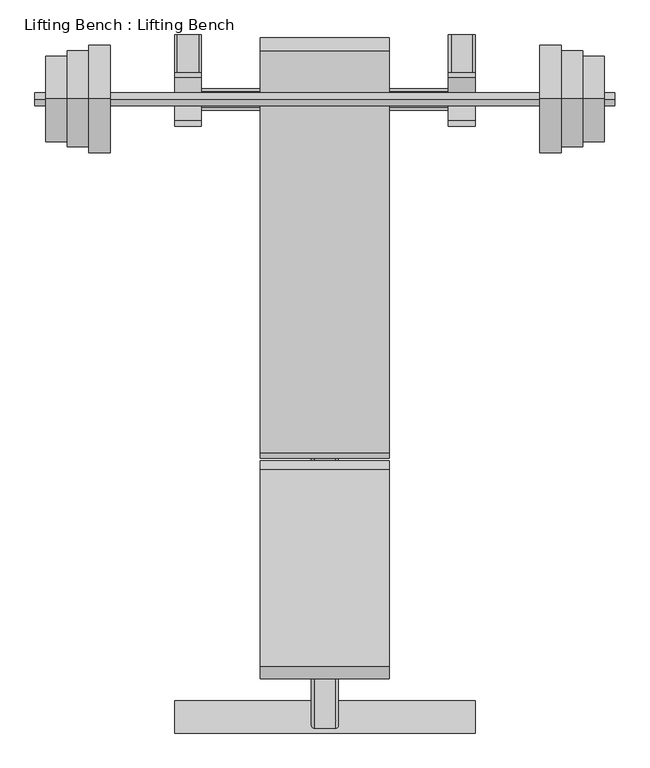
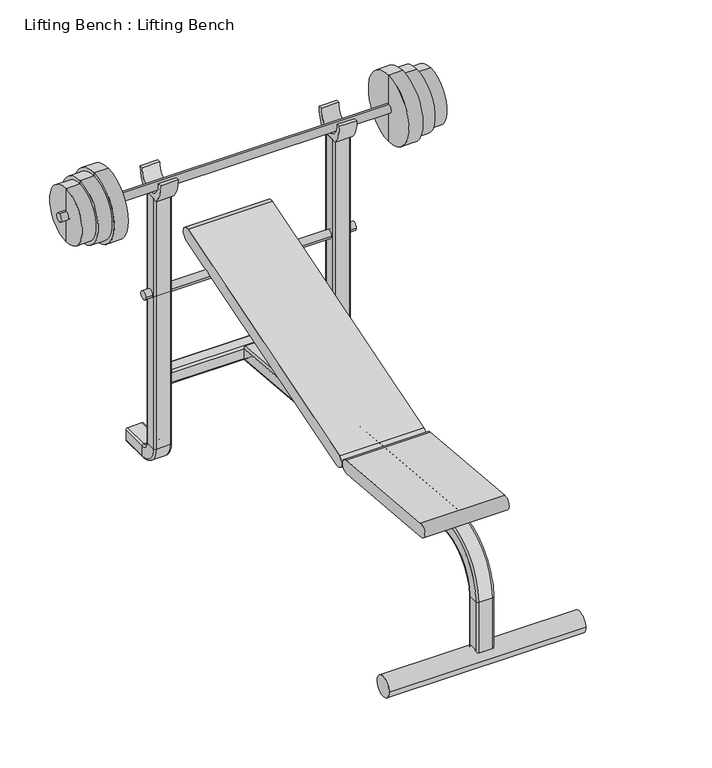
"""IFC4 building model written with IfcOpenShell, lengths in millimetres: proxy geometry, Lifting Bench : Lifting Bench."""

from ifc_helpers import new_model, si_unit, point, frame, frame_2d, origin, place, context, project, spatial, polyline, circle_curve, ellipse_curve, trimmed, segment, composite_curve, outline, extrude, source, transform, mapped, element, save
from ifc_brep_helpers import plane_surface, cylinder_surface, revolved_surface, advanced_brep


def lifting_bench_lifting_bench_243d69f3(model_context):
    return source(origin(), model_context, "Body", "SolidModel", [
        extrude(outline(composite_curve([segment(trimmed(circle_curve(frame_2d((38.1, 39.9587999)), 38.1), [point((0.0, 39.9587999))], [point((76.2, 39.9587999))], False, "CARTESIAN"), True, "CONTINUOUS"), segment(trimmed(circle_curve(frame_2d((38.1, 39.9587999)), 38.1), [point((76.2, 39.9587999))], [point((0.0, 39.9587999))], False, "CARTESIAN"), True, "CONTINUOUS")], self_intersect=False)), frame((0.0, 0.0, 0.0), z_axis=(1.0, 0.0, 0.0), x_axis=(0.0, 1.0, 0.0)), (0.0, 0.0, 1.0), 711.2),
        advanced_brep(
        [(57.15, 1524.0, 1033.9133719), (6.35, 1524.0, 1033.9133719), (0.0, 1517.65, 1033.9133719), (0.0, 1479.55, 1033.9133719), (6.35, 1473.2, 1033.9133719), (57.15, 1473.2, 1033.9133719), (63.5, 1479.55, 1033.9133719), (63.5, 1517.65, 1033.9133719), (57.15, 1524.0, 76.2), (6.35, 1524.0, 76.2), (0.0, 1517.65, 76.2), (0.0, 1479.55, 76.2), (6.35, 1473.2, 76.2), (57.15, 1473.2, 76.2), (63.5, 1479.55, 76.2), (63.5, 1517.65, 76.2), (6.35, 1549.4, 50.8), (57.15, 1549.4, 50.8), (0.0, 1549.4, 44.45), (0.0, 1549.4, 6.35), (6.35, 1549.4, 0.0), (57.15, 1549.4, 0.0), (63.5, 1549.4, 6.35), (63.5, 1549.4, 44.45), (57.15, 1651.0, 50.8), (63.5, 1651.0, 44.45), (63.5, 1651.0, 6.35), (57.15, 1651.0, 0.0), (6.35, 1651.0, 0.0), (0.0, 1651.0, 6.35), (0.0, 1651.0, 44.45), (6.35, 1651.0, 50.8)],
        [
            (0, 1),
            (1, 2, circle_curve(frame((6.35, 1517.65, 1033.9133719), z_axis=(0.0, 0.0, 1.0), x_axis=(1.0, 0.0, 0.0)), 6.35)),
            (2, 3),
            (3, 4, circle_curve(frame((6.35, 1479.55, 1033.9133719), z_axis=(0.0, 0.0, 1.0), x_axis=(1.0, 0.0, 0.0)), 6.35)),
            (4, 5),
            (5, 6, circle_curve(frame((57.15, 1479.55, 1033.9133719), z_axis=(0.0, 0.0, 1.0), x_axis=(1.0, 0.0, 0.0)), 6.35)),
            (6, 7),
            (7, 0, circle_curve(frame((57.15, 1517.65, 1033.9133719), z_axis=(0.0, 0.0, 1.0), x_axis=(1.0, 0.0, 0.0)), 6.35)),
            (0, 8),
            (8, 9),
            (9, 1),
            (9, 10, circle_curve(frame((6.35, 1517.65, 76.2), z_axis=(0.0, 0.0, 1.0), x_axis=(1.0, 0.0, 0.0)), 6.35)),
            (10, 2),
            (10, 11),
            (11, 3),
            (11, 12, circle_curve(frame((6.35, 1479.55, 76.2), z_axis=(0.0, 0.0, 1.0), x_axis=(1.0, 0.0, 0.0)), 6.35)),
            (12, 4),
            (12, 13),
            (13, 5),
            (13, 14, circle_curve(frame((57.15, 1479.55, 76.2), z_axis=(0.0, 0.0, 1.0), x_axis=(1.0, 0.0, 0.0)), 6.35)),
            (14, 6),
            (14, 15),
            (15, 7),
            (15, 8, circle_curve(frame((57.15, 1517.65, 76.2), z_axis=(0.0, 0.0, 1.0), x_axis=(1.0, 0.0, 0.0)), 6.35)),
            (16, 9, circle_curve(frame((6.35, 1549.4, 76.2), z_axis=(-1.0, 0.0, 0.0), x_axis=(0.0, -1.0, 0.0)), 25.4)),
            (8, 17, circle_curve(frame((57.15, 1549.4, 76.2), z_axis=(1.0, 0.0, 0.0), x_axis=(0.0, -1.0, 0.0)), 25.4)),
            (17, 16),
            (18, 10, circle_curve(frame((0.0, 1549.4, 76.2), z_axis=(-1.0, 0.0, 0.0), x_axis=(0.0, -1.0, 0.0)), 31.75)),
            (16, 18, circle_curve(frame((6.35, 1549.4, 44.45), z_axis=(0.0, -1.0, 0.0), x_axis=(1.0, 0.0, 0.0)), 6.35)),
            (19, 11, circle_curve(frame((0.0, 1549.4, 76.2), z_axis=(-1.0, 0.0, 0.0), x_axis=(0.0, -1.0, 0.0)), 69.85)),
            (18, 19),
            (20, 12, circle_curve(frame((6.35, 1549.4, 76.2), z_axis=(-1.0, 0.0, 0.0), x_axis=(0.0, -1.0, 0.0)), 76.2)),
            (19, 20, circle_curve(frame((6.35, 1549.4, 6.35), z_axis=(0.0, -1.0, 0.0), x_axis=(1.0, 0.0, 0.0)), 6.35)),
            (21, 13, circle_curve(frame((57.15, 1549.4, 76.2), z_axis=(-1.0, 0.0, 0.0), x_axis=(0.0, -1.0, 0.0)), 76.2)),
            (20, 21),
            (22, 14, circle_curve(frame((63.5, 1549.4, 76.2), z_axis=(-1.0, 0.0, 0.0), x_axis=(0.0, -1.0, 0.0)), 69.85)),
            (21, 22, circle_curve(frame((57.15, 1549.4, 6.35), z_axis=(0.0, -1.0, 0.0), x_axis=(1.0, 0.0, 0.0)), 6.35)),
            (23, 15, circle_curve(frame((63.5, 1549.4, 76.2), z_axis=(-1.0, 0.0, 0.0), x_axis=(0.0, -1.0, 0.0)), 31.75)),
            (22, 23),
            (23, 17, circle_curve(frame((57.15, 1549.4, 44.45), z_axis=(0.0, -1.0, 0.0), x_axis=(1.0, 0.0, 0.0)), 6.35)),
            (24, 25, circle_curve(frame((57.15, 1651.0, 44.45), z_axis=(0.0, 1.0, 0.0), x_axis=(1.0, 0.0, 0.0)), 6.35)),
            (25, 26),
            (26, 27, circle_curve(frame((57.15, 1651.0, 6.35), z_axis=(0.0, 1.0, 0.0), x_axis=(1.0, 0.0, 0.0)), 6.35)),
            (27, 28),
            (28, 29, circle_curve(frame((6.35, 1651.0, 6.35), z_axis=(0.0, 1.0, 0.0), x_axis=(1.0, 0.0, 0.0)), 6.35)),
            (29, 30),
            (30, 31, circle_curve(frame((6.35, 1651.0, 44.45), z_axis=(0.0, 1.0, 0.0), x_axis=(1.0, 0.0, 0.0)), 6.35)),
            (31, 24),
            (17, 24),
            (31, 16),
            (30, 18),
            (29, 19),
            (28, 20),
            (27, 21),
            (26, 22),
            (25, 23),
        ],
        [
            plane_surface(frame((0.0, 1445.293955, 1033.9133719), z_axis=(0.0, 0.0, 1.0), x_axis=(-1.0, 0.0, 0.0))),
            plane_surface(frame((57.15, 1524.0, 1033.9133719), z_axis=(0.0, 1.0, 0.0), x_axis=(0.0, 0.0, -1.0))),
            cylinder_surface(frame((6.35, 1517.65, 1033.9133719), z_axis=(0.0, 0.0, 1.0), x_axis=(1.0, 0.0, 0.0)), 6.35),
            plane_surface(frame((0.0, 1517.65, 1033.9133719), z_axis=(-1.0, 0.0, 0.0), x_axis=(0.0, 0.0, -1.0))),
            cylinder_surface(frame((6.35, 1479.55, 1033.9133719), z_axis=(0.0, 0.0, 1.0), x_axis=(1.0, 0.0, 0.0)), 6.35),
            plane_surface(frame((6.35, 1473.2, 1033.9133719), z_axis=(0.0, -1.0, 0.0), x_axis=(0.0, 0.0, -1.0))),
            cylinder_surface(frame((57.15, 1479.55, 1033.9133719), z_axis=(0.0, 0.0, 1.0), x_axis=(1.0, 0.0, 0.0)), 6.35),
            plane_surface(frame((63.5, 1479.55, 1033.9133719), z_axis=(1.0, 0.0, 0.0), x_axis=(0.0, 0.0, -1.0))),
            cylinder_surface(frame((57.15, 1517.65, 1033.9133719), z_axis=(0.0, 0.0, 1.0), x_axis=(1.0, 0.0, 0.0)), 6.35),
            revolved_surface(polyline([(57.15, 1524.0, 76.2), (6.35, 1524.0, 76.2)]), (0.0, 1549.4, 76.2), (1.0, 0.0, 0.0)),
            revolved_surface(trimmed(ellipse_curve(frame((6.35, 1517.65, 76.2), z_axis=(0.0, 0.0, 1.0), x_axis=(1.0, 0.0, 0.0)), 6.35, 6.35), [point((6.35, 1524.0, 76.2))], [point((0.0, 1517.65, 76.2))], True, "CARTESIAN"), (0.0, 1549.4, 76.2), (1.0, 0.0, 0.0)),
            plane_surface(frame((0.0, 1549.4, 76.2), z_axis=(-1.0, 0.0, 0.0), x_axis=(0.0, -1.0, 0.0))),
            revolved_surface(trimmed(ellipse_curve(frame((6.35, 1479.55, 76.2), z_axis=(0.0, 0.0, 1.0), x_axis=(1.0, 0.0, 0.0)), 6.35, 6.35), [point((0.0, 1479.55, 76.2))], [point((6.35, 1473.2, 76.2))], True, "CARTESIAN"), (0.0, 1549.4, 76.2), (1.0, 0.0, 0.0)),
            cylinder_surface(frame((0.0, 1549.4, 76.2), z_axis=(1.0, 0.0, 0.0), x_axis=(0.0, -1.0, 0.0)), 76.2),
            revolved_surface(trimmed(ellipse_curve(frame((57.15, 1479.55, 76.2), z_axis=(0.0, 0.0, 1.0), x_axis=(1.0, 0.0, 0.0)), 6.35, 6.35), [point((57.15, 1473.2, 76.2))], [point((63.5, 1479.55, 76.2))], True, "CARTESIAN"), (0.0, 1549.4, 76.2), (1.0, 0.0, 0.0)),
            plane_surface(frame((63.5, 1549.4, 76.2), z_axis=(1.0, 0.0, 0.0), x_axis=(0.0, -1.0, 0.0))),
            revolved_surface(trimmed(ellipse_curve(frame((57.15, 1517.65, 76.2), z_axis=(0.0, 0.0, 1.0), x_axis=(1.0, 0.0, 0.0)), 6.35, 6.35), [point((63.5, 1517.65, 76.2))], [point((57.15, 1524.0, 76.2))], True, "CARTESIAN"), (0.0, 1549.4, 76.2), (1.0, 0.0, 0.0)),
            plane_surface(frame((-78.706045, 1651.0, 50.8), z_axis=(0.0, 1.0, 0.0), x_axis=(0.0, 0.0, 1.0))),
            plane_surface(frame((57.15, 1549.4, 50.8), z_axis=(0.0, 0.0, 1.0), x_axis=(0.0, 1.0, 0.0))),
            cylinder_surface(frame((6.35, 1549.4, 44.45), z_axis=(0.0, -1.0, 0.0), x_axis=(1.0, 0.0, 0.0)), 6.35),
            plane_surface(frame((0.0, 1549.4, 44.45), z_axis=(-1.0, 0.0, 0.0), x_axis=(0.0, 1.0, 0.0))),
            cylinder_surface(frame((6.35, 1549.4, 6.35), z_axis=(0.0, -1.0, 0.0), x_axis=(1.0, 0.0, 0.0)), 6.35),
            plane_surface(frame((6.35, 1549.4, 0.0), z_axis=(0.0, 0.0, -1.0), x_axis=(0.0, 1.0, 0.0))),
            cylinder_surface(frame((57.15, 1549.4, 6.35), z_axis=(0.0, -1.0, 0.0), x_axis=(1.0, 0.0, 0.0)), 6.35),
            plane_surface(frame((63.5, 1549.4, 6.35), z_axis=(1.0, 0.0, 0.0), x_axis=(0.0, 1.0, 0.0))),
            cylinder_surface(frame((57.15, 1549.4, 44.45), z_axis=(0.0, -1.0, 0.0), x_axis=(1.0, 0.0, 0.0)), 6.35),
        ],
        [
            (0, [[1, 2, 3, 4, 5, 6, 7, 8]]),
            (1, [[-1, 9, 10, 11]]),
            (2, [[-2, -11, 12, 13]]),
            (3, [[-3, -13, 14, 15]]),
            (4, [[-4, -15, 16, 17]]),
            (5, [[-5, -17, 18, 19]]),
            (6, [[-6, -19, 20, 21]]),
            (7, [[-7, -21, 22, 23]]),
            (8, [[-8, -23, 24, -9]]),
            (9, [[25, -10, 26, 27]]),
            (10, [[28, -12, -25, 29]]),
            (11, [[30, -14, -28, 31]]),
            (12, [[32, -16, -30, 33]]),
            (13, [[34, -18, -32, 35]]),
            (14, [[36, -20, -34, 37]]),
            (15, [[38, -22, -36, 39]]),
            (16, [[-26, -24, -38, 40]]),
            (17, [[41, 42, 43, 44, 45, 46, 47, 48]]),
            (18, [[-27, 49, -48, 50]]),
            (19, [[-29, -50, -47, 51]]),
            (20, [[-31, -51, -46, 52]]),
            (21, [[-33, -52, -45, 53]]),
            (22, [[-35, -53, -44, 54]]),
            (23, [[-37, -54, -43, 55]]),
            (24, [[-39, -55, -42, 56]]),
            (25, [[-40, -56, -41, -49]]),
        ],
    ),
        advanced_brep(
        [(654.05, 1524.0, 1033.9133719), (647.7, 1517.65, 1033.9133719), (647.7, 1479.55, 1033.9133719), (654.05, 1473.2, 1033.9133719), (704.85, 1473.2, 1033.9133719), (711.2, 1479.55, 1033.9133719), (711.2, 1517.65, 1033.9133719), (704.85, 1524.0, 1033.9133719), (654.05, 1524.0, 76.2), (647.7, 1517.65, 76.2), (647.7, 1479.55, 76.2), (654.05, 1473.2, 76.2), (704.85, 1473.2, 76.2), (711.2, 1479.55, 76.2), (711.2, 1517.65, 76.2), (704.85, 1524.0, 76.2), (647.7, 1549.4, 44.45), (654.05, 1549.4, 50.8), (647.7, 1549.4, 6.35), (654.05, 1549.4, 0.0), (704.85, 1549.4, 0.0), (711.2, 1549.4, 6.35), (711.2, 1549.4, 44.45), (704.85, 1549.4, 50.8), (654.05, 1651.0, 50.8), (704.85, 1651.0, 50.8), (711.2, 1651.0, 44.45), (711.2, 1651.0, 6.35), (704.85, 1651.0, 0.0), (654.05, 1651.0, 0.0), (647.7, 1651.0, 6.35), (647.7, 1651.0, 44.45)],
        [
            (0, 1, circle_curve(frame((654.05, 1517.65, 1033.9133719), z_axis=(0.0, 0.0, 1.0), x_axis=(-1.0, 0.0, 0.0)), 6.35)),
            (1, 2),
            (2, 3, circle_curve(frame((654.05, 1479.55, 1033.9133719), z_axis=(0.0, 0.0, 1.0), x_axis=(-1.0, 0.0, 0.0)), 6.35)),
            (3, 4),
            (4, 5, circle_curve(frame((704.85, 1479.55, 1033.9133719), z_axis=(0.0, 0.0, 1.0), x_axis=(-1.0, 0.0, 0.0)), 6.35)),
            (5, 6),
            (6, 7, circle_curve(frame((704.85, 1517.65, 1033.9133719), z_axis=(0.0, 0.0, 1.0), x_axis=(-1.0, 0.0, 0.0)), 6.35)),
            (7, 0),
            (0, 8),
            (8, 9, circle_curve(frame((654.05, 1517.65, 76.2), z_axis=(0.0, 0.0, 1.0), x_axis=(-1.0, 0.0, 0.0)), 6.35)),
            (9, 1),
            (9, 10),
            (10, 2),
            (10, 11, circle_curve(frame((654.05, 1479.55, 76.2), z_axis=(0.0, 0.0, 1.0), x_axis=(-1.0, 0.0, 0.0)), 6.35)),
            (11, 3),
            (11, 12),
            (12, 4),
            (12, 13, circle_curve(frame((704.85, 1479.55, 76.2), z_axis=(0.0, 0.0, 1.0), x_axis=(-1.0, 0.0, 0.0)), 6.35)),
            (13, 5),
            (13, 14),
            (14, 6),
            (14, 15, circle_curve(frame((704.85, 1517.65, 76.2), z_axis=(0.0, 0.0, 1.0), x_axis=(-1.0, 0.0, 0.0)), 6.35)),
            (15, 7),
            (15, 8),
            (16, 9, circle_curve(frame((647.7, 1549.4, 76.2), z_axis=(-1.0, 0.0, 0.0), x_axis=(0.0, -1.0, 0.0)), 31.75)),
            (8, 17, circle_curve(frame((654.05, 1549.4, 76.2), z_axis=(1.0, 0.0, 0.0), x_axis=(0.0, -1.0, 0.0)), 25.4)),
            (17, 16, circle_curve(frame((654.05, 1549.4, 44.45), z_axis=(0.0, -1.0, 0.0), x_axis=(-1.0, 0.0, 0.0)), 6.35)),
            (18, 10, circle_curve(frame((647.7, 1549.4, 76.2), z_axis=(-1.0, 0.0, 0.0), x_axis=(0.0, -1.0, 0.0)), 69.85)),
            (16, 18),
            (19, 11, circle_curve(frame((654.05, 1549.4, 76.2), z_axis=(-1.0, 0.0, 0.0), x_axis=(0.0, -1.0, 0.0)), 76.2)),
            (18, 19, circle_curve(frame((654.05, 1549.4, 6.35), z_axis=(0.0, -1.0, 0.0), x_axis=(-1.0, 0.0, 0.0)), 6.35)),
            (20, 12, circle_curve(frame((704.85, 1549.4, 76.2), z_axis=(-1.0, 0.0, 0.0), x_axis=(0.0, -1.0, 0.0)), 76.2)),
            (19, 20),
            (21, 13, circle_curve(frame((711.2, 1549.4, 76.2), z_axis=(-1.0, 0.0, 0.0), x_axis=(0.0, -1.0, 0.0)), 69.85)),
            (20, 21, circle_curve(frame((704.85, 1549.4, 6.35), z_axis=(0.0, -1.0, 0.0), x_axis=(-1.0, 0.0, 0.0)), 6.35)),
            (22, 14, circle_curve(frame((711.2, 1549.4, 76.2), z_axis=(-1.0, 0.0, 0.0), x_axis=(0.0, -1.0, 0.0)), 31.75)),
            (21, 22),
            (23, 15, circle_curve(frame((704.85, 1549.4, 76.2), z_axis=(-1.0, 0.0, 0.0), x_axis=(0.0, -1.0, 0.0)), 25.4)),
            (22, 23, circle_curve(frame((704.85, 1549.4, 44.45), z_axis=(0.0, -1.0, 0.0), x_axis=(-1.0, 0.0, 0.0)), 6.35)),
            (23, 17),
            (24, 25),
            (25, 26, circle_curve(frame((704.85, 1651.0, 44.45), z_axis=(0.0, 1.0, 0.0), x_axis=(-1.0, 0.0, 0.0)), 6.35)),
            (26, 27),
            (27, 28, circle_curve(frame((704.85, 1651.0, 6.35), z_axis=(0.0, 1.0, 0.0), x_axis=(-1.0, 0.0, 0.0)), 6.35)),
            (28, 29),
            (29, 30, circle_curve(frame((654.05, 1651.0, 6.35), z_axis=(0.0, 1.0, 0.0), x_axis=(-1.0, 0.0, 0.0)), 6.35)),
            (30, 31),
            (31, 24, circle_curve(frame((654.05, 1651.0, 44.45), z_axis=(0.0, 1.0, 0.0), x_axis=(-1.0, 0.0, 0.0)), 6.35)),
            (17, 24),
            (31, 16),
            (30, 18),
            (29, 19),
            (28, 20),
            (27, 21),
            (26, 22),
            (25, 23),
        ],
        [
            plane_surface(frame((711.2, 1445.293955, 1033.9133719), z_axis=(0.0, 0.0, 1.0), x_axis=(-1.0, 0.0, 0.0))),
            cylinder_surface(frame((654.05, 1517.65, 1033.9133719), z_axis=(0.0, 0.0, 1.0), x_axis=(-1.0, 0.0, 0.0)), 6.35),
            plane_surface(frame((647.7, 1517.65, 1033.9133719), z_axis=(-1.0, 0.0, 0.0), x_axis=(0.0, 0.0, -1.0))),
            cylinder_surface(frame((654.05, 1479.55, 1033.9133719), z_axis=(0.0, 0.0, 1.0), x_axis=(-1.0, 0.0, 0.0)), 6.35),
            plane_surface(frame((654.05, 1473.2, 1033.9133719), z_axis=(0.0, -1.0, 0.0), x_axis=(0.0, 0.0, -1.0))),
            cylinder_surface(frame((704.85, 1479.55, 1033.9133719), z_axis=(0.0, 0.0, 1.0), x_axis=(-1.0, 0.0, 0.0)), 6.35),
            plane_surface(frame((711.2, 1479.55, 1033.9133719), z_axis=(1.0, 0.0, 0.0), x_axis=(0.0, 0.0, -1.0))),
            cylinder_surface(frame((704.85, 1517.65, 1033.9133719), z_axis=(0.0, 0.0, 1.0), x_axis=(-1.0, 0.0, 0.0)), 6.35),
            plane_surface(frame((704.85, 1524.0, 1033.9133719), z_axis=(0.0, 1.0, 0.0), x_axis=(0.0, 0.0, -1.0))),
            revolved_surface(trimmed(ellipse_curve(frame((654.05, 1517.65, 76.2), z_axis=(0.0, 0.0, 1.0), x_axis=(-1.0, 0.0, 0.0)), 6.35, 6.35), [point((654.05, 1524.0, 76.2))], [point((647.7, 1517.65, 76.2))], True, "CARTESIAN"), (711.2, 1549.4, 76.2), (1.0, 0.0, 0.0)),
            plane_surface(frame((647.7, 1549.4, 76.2), z_axis=(-1.0, 0.0, 0.0), x_axis=(0.0, -1.0, 0.0))),
            revolved_surface(trimmed(ellipse_curve(frame((654.05, 1479.55, 76.2), z_axis=(0.0, 0.0, 1.0), x_axis=(-1.0, 0.0, 0.0)), 6.35, 6.35), [point((647.7, 1479.55, 76.2))], [point((654.05, 1473.2, 76.2))], True, "CARTESIAN"), (711.2, 1549.4, 76.2), (1.0, 0.0, 0.0)),
            cylinder_surface(frame((711.2, 1549.4, 76.2), z_axis=(1.0, 0.0, 0.0), x_axis=(0.0, -1.0, 0.0)), 76.2),
            revolved_surface(trimmed(ellipse_curve(frame((704.85, 1479.55, 76.2), z_axis=(0.0, 0.0, 1.0), x_axis=(-1.0, 0.0, 0.0)), 6.35, 6.35), [point((704.85, 1473.2, 76.2))], [point((711.2, 1479.55, 76.2))], True, "CARTESIAN"), (711.2, 1549.4, 76.2), (1.0, 0.0, 0.0)),
            plane_surface(frame((711.2, 1549.4, 76.2), z_axis=(1.0, 0.0, 0.0), x_axis=(0.0, -1.0, 0.0))),
            revolved_surface(trimmed(ellipse_curve(frame((704.85, 1517.65, 76.2), z_axis=(0.0, 0.0, 1.0), x_axis=(-1.0, 0.0, 0.0)), 6.35, 6.35), [point((711.2, 1517.65, 76.2))], [point((704.85, 1524.0, 76.2))], True, "CARTESIAN"), (711.2, 1549.4, 76.2), (1.0, 0.0, 0.0)),
            revolved_surface(polyline([(704.85, 1524.0, 76.2), (654.05, 1524.0, 76.2)]), (711.2, 1549.4, 76.2), (1.0, 0.0, 0.0)),
            plane_surface(frame((632.493955, 1651.0, 50.8), z_axis=(0.0, 1.0, 0.0), x_axis=(0.0, 0.0, 1.0))),
            cylinder_surface(frame((654.05, 1549.4, 44.45), z_axis=(0.0, -1.0, 0.0), x_axis=(-1.0, 0.0, 0.0)), 6.35),
            plane_surface(frame((647.7, 1549.4, 44.45), z_axis=(-1.0, 0.0, 0.0), x_axis=(0.0, 1.0, 0.0))),
            cylinder_surface(frame((654.05, 1549.4, 6.35), z_axis=(0.0, -1.0, 0.0), x_axis=(-1.0, 0.0, 0.0)), 6.35),
            plane_surface(frame((654.05, 1549.4, 0.0), z_axis=(0.0, 0.0, -1.0), x_axis=(0.0, 1.0, 0.0))),
            cylinder_surface(frame((704.85, 1549.4, 6.35), z_axis=(0.0, -1.0, 0.0), x_axis=(-1.0, 0.0, 0.0)), 6.35),
            plane_surface(frame((711.2, 1549.4, 6.35), z_axis=(1.0, 0.0, 0.0), x_axis=(0.0, 1.0, 0.0))),
            cylinder_surface(frame((704.85, 1549.4, 44.45), z_axis=(0.0, -1.0, 0.0), x_axis=(-1.0, 0.0, 0.0)), 6.35),
            plane_surface(frame((704.85, 1549.4, 50.8), z_axis=(0.0, 0.0, 1.0), x_axis=(0.0, 1.0, 0.0))),
        ],
        [
            (0, [[1, 2, 3, 4, 5, 6, 7, 8]]),
            (1, [[-1, 9, 10, 11]]),
            (2, [[-2, -11, 12, 13]]),
            (3, [[-3, -13, 14, 15]]),
            (4, [[-4, -15, 16, 17]]),
            (5, [[-5, -17, 18, 19]]),
            (6, [[-6, -19, 20, 21]]),
            (7, [[-7, -21, 22, 23]]),
            (8, [[-8, -23, 24, -9]]),
            (9, [[25, -10, 26, 27]]),
            (10, [[28, -12, -25, 29]]),
            (11, [[30, -14, -28, 31]]),
            (12, [[32, -16, -30, 33]]),
            (13, [[34, -18, -32, 35]]),
            (14, [[36, -20, -34, 37]]),
            (15, [[38, -22, -36, 39]]),
            (16, [[-26, -24, -38, 40]]),
            (17, [[41, 42, 43, 44, 45, 46, 47, 48]]),
            (18, [[-27, 49, -48, 50]]),
            (19, [[-29, -50, -47, 51]]),
            (20, [[-31, -51, -46, 52]]),
            (21, [[-33, -52, -45, 53]]),
            (22, [[-35, -53, -44, 54]]),
            (23, [[-37, -54, -43, 55]]),
            (24, [[-39, -55, -42, 56]]),
            (25, [[-40, -56, -41, -49]]),
        ],
    ),
        extrude(outline(composite_curve([segment(trimmed(circle_curve(frame_2d((1479.55, 311.15)), 6.35), [point((1479.55, 304.8))], [point((1473.2, 311.15))], False, "CARTESIAN"), True, "CONTINUOUS"), segment(polyline([(1473.2, 311.15), (1473.2, 349.25)]), True, "CONTINUOUS"), segment(trimmed(circle_curve(frame_2d((1479.55, 349.25)), 6.35), [point((1473.2, 349.25))], [point((1479.55, 355.6))], False, "CARTESIAN"), True, "CONTINUOUS"), segment(polyline([(1479.55, 355.6), (1517.65, 355.6)]), True, "CONTINUOUS"), segment(trimmed(circle_curve(frame_2d((1517.65, 349.25)), 6.35), [point((1517.65, 355.6))], [point((1524.0, 349.25))], False, "CARTESIAN"), True, "CONTINUOUS"), segment(polyline([(1524.0, 349.25), (1524.0, 311.15)]), True, "CONTINUOUS"), segment(trimmed(circle_curve(frame_2d((1517.65, 311.15)), 6.35), [point((1524.0, 311.15))], [point((1517.65, 304.8))], False, "CARTESIAN"), True, "CONTINUOUS"), segment(polyline([(1517.65, 304.8), (1479.55, 304.8)]), True, "CONTINUOUS")], self_intersect=False)), frame((63.5, 0.0, 0.0), z_axis=(1.0, 0.0, 0.0), x_axis=(0.0, 1.0, 0.0)), (0.0, 0.0, 1.0), 584.2),
        advanced_brep(
        [(381.0, 1482.8987076, 355.0170142), (387.35, 1482.3452686, 348.6911779), (387.35, 1479.0246348, 310.7361599), (381.0, 1478.4711959, 304.4103235), (330.2, 1478.4711959, 304.4103235), (323.85, 1479.0246348, 310.7361599), (323.85, 1482.3452686, 348.6911779), (330.2, 1482.8987076, 355.0170142), (381.0, 231.9876606, 464.4575499), (387.35, 231.4342216, 458.1317136), (387.35, 228.1135878, 420.1766956), (381.0, 227.5601489, 413.8508592), (330.2, 227.5601489, 413.8508592), (323.85, 228.1135878, 420.1766956), (323.85, 231.4342216, 458.1317136), (330.2, 231.9876606, 464.4575499), (387.35, 17.958351, 262.5171184), (381.0, 11.608351, 262.5171184), (387.35, 56.058351, 262.5171184), (381.0, 62.408351, 262.5171184), (330.2, 62.408351, 262.5171184), (323.85, 56.058351, 262.5171184), (323.85, 17.958351, 262.5171184), (330.2, 11.608351, 262.5171184), (381.0, 11.608351, 40.4636494), (330.2, 11.608351, 40.4636494), (323.85, 17.958351, 40.4636494), (323.85, 56.058351, 40.4636494), (330.2, 62.408351, 40.4636494), (381.0, 62.408351, 40.4636494), (387.35, 56.058351, 40.4636494), (387.35, 17.958351, 40.4636494)],
        [
            (0, 1, circle_curve(frame((381.0, 1482.3452686, 348.6911779), z_axis=(0.0, 0.9961946980917459, -0.08715574274765438), x_axis=(0.0, 0.08715574274765438, 0.9961946980917459)), 6.35)),
            (1, 2),
            (2, 3, circle_curve(frame((381.0, 1479.0246348, 310.7361599), z_axis=(0.0, 0.9961946980917459, -0.08715574274765438), x_axis=(0.0, 0.08715574274765438, 0.9961946980917459)), 6.35)),
            (3, 4),
            (4, 5, circle_curve(frame((330.2, 1479.0246348, 310.7361599), z_axis=(0.0, 0.9961946980917459, -0.08715574274765438), x_axis=(0.0, 0.08715574274765438, 0.9961946980917459)), 6.35)),
            (5, 6),
            (6, 7, circle_curve(frame((330.2, 1482.3452686, 348.6911779), z_axis=(0.0, 0.9961946980917459, -0.08715574274765438), x_axis=(0.0, 0.08715574274765438, 0.9961946980917459)), 6.35)),
            (7, 0),
            (0, 8),
            (8, 9, circle_curve(frame((381.0, 231.4342216, 458.1317136), z_axis=(0.0, 0.9961946980917459, -0.08715574274765438), x_axis=(0.0, 0.08715574274765438, 0.9961946980917459)), 6.35)),
            (9, 1),
            (9, 10),
            (10, 2),
            (10, 11, circle_curve(frame((381.0, 228.1135878, 420.1766956), z_axis=(0.0, 0.9961946980917459, -0.08715574274765438), x_axis=(0.0, 0.08715574274765438, 0.9961946980917459)), 6.35)),
            (11, 3),
            (11, 12),
            (12, 4),
            (12, 13, circle_curve(frame((330.2, 228.1135878, 420.1766956), z_axis=(0.0, 0.9961946980917459, -0.08715574274765438), x_axis=(0.0, 0.08715574274765438, 0.9961946980917459)), 6.35)),
            (13, 5),
            (13, 14),
            (14, 6),
            (14, 15, circle_curve(frame((330.2, 231.4342216, 458.1317136), z_axis=(0.0, 0.9961946980917459, -0.08715574274765438), x_axis=(0.0, 0.08715574274765438, 0.9961946980917459)), 6.35)),
            (15, 7),
            (15, 8),
            (16, 9, circle_curve(frame((387.35, 214.3201621, 262.5171184), z_axis=(-1.0, 0.0, 0.0), x_axis=(0.0, 0.08715574274765332, 0.996194698091746)), 196.3618112)),
            (8, 17, circle_curve(frame((381.0, 214.3201621, 262.5171184), z_axis=(1.0, 0.0, 0.0), x_axis=(0.0, 0.08715574274765332, 0.996194698091746)), 202.7118112)),
            (17, 16, circle_curve(frame((381.0, 17.958351, 262.5171184), z_axis=(0.0, 0.0, 1.0000000000000002), x_axis=(0.0, -1.0000000000000002, 0.0)), 6.35)),
            (18, 10, circle_curve(frame((387.35, 214.3201621, 262.5171184), z_axis=(-1.0, 0.0, 0.0), x_axis=(0.0, 0.08715574274765332, 0.996194698091746)), 158.2618112)),
            (16, 18),
            (19, 11, circle_curve(frame((381.0, 214.3201621, 262.5171184), z_axis=(-1.0, 0.0, 0.0), x_axis=(0.0, 0.08715574274765332, 0.996194698091746)), 151.9118112)),
            (18, 19, circle_curve(frame((381.0, 56.058351, 262.5171184), z_axis=(0.0, 0.0, 1.0000000000000002), x_axis=(0.0, -1.0000000000000002, 0.0)), 6.35)),
            (20, 12, circle_curve(frame((330.2, 214.3201621, 262.5171184), z_axis=(-1.0, 0.0, 0.0), x_axis=(0.0, 0.08715574274765332, 0.996194698091746)), 151.9118112)),
            (19, 20),
            (21, 13, circle_curve(frame((323.85, 214.3201621, 262.5171184), z_axis=(-1.0, 0.0, 0.0), x_axis=(0.0, 0.08715574274765332, 0.996194698091746)), 158.2618112)),
            (20, 21, circle_curve(frame((330.2, 56.058351, 262.5171184), z_axis=(0.0, 0.0, 1.0000000000000002), x_axis=(0.0, -1.0000000000000002, 0.0)), 6.35)),
            (22, 14, circle_curve(frame((323.85, 214.3201621, 262.5171184), z_axis=(-1.0, 0.0, 0.0), x_axis=(0.0, 0.08715574274765332, 0.996194698091746)), 196.3618112)),
            (21, 22),
            (23, 15, circle_curve(frame((330.2, 214.3201621, 262.5171184), z_axis=(-1.0, 0.0, 0.0), x_axis=(0.0, 0.08715574274765332, 0.996194698091746)), 202.7118112)),
            (22, 23, circle_curve(frame((330.2, 17.958351, 262.5171184), z_axis=(0.0, 0.0, 1.0000000000000002), x_axis=(0.0, -1.0000000000000002, 0.0)), 6.35)),
            (23, 17),
            (24, 25),
            (25, 26, circle_curve(frame((330.2, 17.958351, 40.4636494), z_axis=(0.0, 0.0, -1.0), x_axis=(0.0, -1.0, 0.0)), 6.35)),
            (26, 27),
            (27, 28, circle_curve(frame((330.2, 56.058351, 40.4636494), z_axis=(0.0, 0.0, -1.0), x_axis=(0.0, -1.0, 0.0)), 6.35)),
            (28, 29),
            (29, 30, circle_curve(frame((381.0, 56.058351, 40.4636494), z_axis=(0.0, 0.0, -1.0), x_axis=(0.0, -1.0, 0.0)), 6.35)),
            (30, 31),
            (31, 24, circle_curve(frame((381.0, 17.958351, 40.4636494), z_axis=(0.0, 0.0, -1.0), x_axis=(0.0, -1.0, 0.0)), 6.35)),
            (17, 24),
            (31, 16),
            (30, 18),
            (29, 19),
            (28, 20),
            (27, 21),
            (26, 22),
            (25, 23),
        ],
        [
            plane_surface(frame((323.85, 1474.9370581, 264.0149443), z_axis=(0.0, 0.996194698091746, -0.08715574274765454), x_axis=(1.0, 0.0, 0.0))),
            cylinder_surface(frame((381.0, 1482.3452686, 348.6911779), z_axis=(0.0, 0.9961946980917459, -0.08715574274765438), x_axis=(0.0, 0.08715574274765438, 0.9961946980917459)), 6.35),
            plane_surface(frame((387.35, 1482.3452686, 348.6911779), z_axis=(1.0000000000000002, 0.0, 0.0), x_axis=(0.0, -0.9961946980917459, 0.08715574274765485))),
            cylinder_surface(frame((381.0, 1479.0246348, 310.7361599), z_axis=(0.0, 0.9961946980917459, -0.08715574274765438), x_axis=(0.0, 0.08715574274765438, 0.9961946980917459)), 6.35),
            plane_surface(frame((381.0, 1478.4711959, 304.4103235), z_axis=(0.0, -0.08715574274765484, -0.9961946980917459), x_axis=(0.0, -0.9961946980917459, 0.08715574274765484))),
            cylinder_surface(frame((330.2, 1479.0246348, 310.7361599), z_axis=(0.0, 0.9961946980917459, -0.08715574274765438), x_axis=(0.0, 0.08715574274765438, 0.9961946980917459)), 6.35),
            plane_surface(frame((323.85, 1479.0246348, 310.7361599), z_axis=(-1.0000000000000002, 0.0, 0.0), x_axis=(0.0, -0.9961946980917459, 0.08715574274765484))),
            cylinder_surface(frame((330.2, 1482.3452686, 348.6911779), z_axis=(0.0, 0.9961946980917459, -0.08715574274765438), x_axis=(0.0, 0.08715574274765438, 0.9961946980917459)), 6.35),
            plane_surface(frame((330.2, 1482.8987076, 355.0170142), z_axis=(0.0, 0.08715574274765484, 0.9961946980917459), x_axis=(0.0, -0.9961946980917459, 0.08715574274765484))),
            revolved_surface(trimmed(ellipse_curve(frame((381.0, 231.4342216, 458.1317136), z_axis=(0.0, 0.996194698091746, -0.08715574274765284), x_axis=(0.0, 0.08715574274765284, 0.996194698091746)), 6.35, 6.35), [point((381.0, 231.9876606, 464.4575499))], [point((387.35, 231.4342216, 458.1317136))], True, "CARTESIAN"), (323.85, 214.3201621, 262.5171184), (1.0, 0.0, 0.0)),
            plane_surface(frame((387.35, 214.3201621, 262.5171184), z_axis=(1.0, 0.0, 0.0), x_axis=(0.0, 0.08715574274765332, 0.996194698091746))),
            revolved_surface(trimmed(ellipse_curve(frame((381.0, 228.1135878, 420.1766956), z_axis=(0.0, 0.996194698091746, -0.08715574274765284), x_axis=(0.0, 0.08715574274765284, 0.996194698091746)), 6.35, 6.35), [point((387.35, 228.1135878, 420.1766956))], [point((381.0, 227.5601489, 413.8508592))], True, "CARTESIAN"), (323.85, 214.3201621, 262.5171184), (1.0, 0.0, 0.0)),
            revolved_surface(polyline([(381.0, 227.5601488372773, 413.8508592949543), (330.2, 227.5601488372773, 413.8508592949543)]), (323.85, 214.3201621, 262.5171184), (1.0, 0.0, 0.0)),
            revolved_surface(trimmed(ellipse_curve(frame((330.2, 228.1135878, 420.1766956), z_axis=(0.0, 0.996194698091746, -0.08715574274765284), x_axis=(0.0, 0.08715574274765284, 0.996194698091746)), 6.35, 6.35), [point((330.2, 227.5601489, 413.8508592))], [point((323.85, 228.1135878, 420.1766956))], True, "CARTESIAN"), (323.85, 214.3201621, 262.5171184), (1.0, 0.0, 0.0)),
            plane_surface(frame((323.85, 214.3201621, 262.5171184), z_axis=(-1.0, 0.0, 0.0), x_axis=(0.0, 0.08715574274765332, 0.996194698091746))),
            revolved_surface(trimmed(ellipse_curve(frame((330.2, 231.4342216, 458.1317136), z_axis=(0.0, 0.996194698091746, -0.08715574274765284), x_axis=(0.0, 0.08715574274765284, 0.996194698091746)), 6.35, 6.35), [point((323.85, 231.4342216, 458.1317136))], [point((330.2, 231.9876606, 464.4575499))], True, "CARTESIAN"), (323.85, 214.3201621, 262.5171184), (1.0, 0.0, 0.0)),
            cylinder_surface(frame((323.85, 214.3201621, 262.5171184), z_axis=(1.0, 0.0, 0.0), x_axis=(0.0, 0.08715574274765332, 0.996194698091746)), 202.7118112),
            plane_surface(frame((323.85, -29.9177098, 40.4636494), z_axis=(0.0, 0.0, -1.0), x_axis=(-1.0, 0.0, 0.0))),
            cylinder_surface(frame((381.0, 17.958351, 262.5171184), z_axis=(0.0, 0.0, 1.0), x_axis=(0.0, -1.0, 0.0)), 6.35),
            plane_surface(frame((387.35, 17.958351, 262.5171184), z_axis=(1.0, 0.0, 0.0), x_axis=(0.0, 0.0, -1.0))),
            cylinder_surface(frame((381.0, 56.058351, 262.5171184), z_axis=(0.0, 0.0, 1.0), x_axis=(0.0, -1.0, 0.0)), 6.35),
            plane_surface(frame((381.0, 62.408351, 262.5171184), z_axis=(0.0, 1.0, 0.0), x_axis=(0.0, 0.0, -1.0))),
            cylinder_surface(frame((330.2, 56.058351, 262.5171184), z_axis=(0.0, 0.0, 1.0), x_axis=(0.0, -1.0, 0.0)), 6.35),
            plane_surface(frame((323.85, 56.058351, 262.5171184), z_axis=(-1.0, 0.0, 0.0), x_axis=(0.0, 0.0, -1.0))),
            cylinder_surface(frame((330.2, 17.958351, 262.5171184), z_axis=(0.0, 0.0, 1.0), x_axis=(0.0, -1.0, 0.0)), 6.35),
            plane_surface(frame((330.2, 11.608351, 262.5171184), z_axis=(0.0, -1.0, 0.0), x_axis=(0.0, 0.0, -1.0))),
        ],
        [
            (0, [[1, 2, 3, 4, 5, 6, 7, 8]]),
            (1, [[-1, 9, 10, 11]]),
            (2, [[-2, -11, 12, 13]]),
            (3, [[-3, -13, 14, 15]]),
            (4, [[-4, -15, 16, 17]]),
            (5, [[-5, -17, 18, 19]]),
            (6, [[-6, -19, 20, 21]]),
            (7, [[-7, -21, 22, 23]]),
            (8, [[-8, -23, 24, -9]]),
            (9, [[25, -10, 26, 27]]),
            (10, [[28, -12, -25, 29]]),
            (11, [[30, -14, -28, 31]]),
            (12, [[32, -16, -30, 33]]),
            (13, [[34, -18, -32, 35]]),
            (14, [[36, -20, -34, 37]]),
            (15, [[38, -22, -36, 39]]),
            (16, [[-26, -24, -38, 40]]),
            (17, [[41, 42, 43, 44, 45, 46, 47, 48]]),
            (18, [[-27, 49, -48, 50]]),
            (19, [[-29, -50, -47, 51]]),
            (20, [[-31, -51, -46, 52]]),
            (21, [[-33, -52, -45, 53]]),
            (22, [[-35, -53, -44, 54]]),
            (23, [[-37, -54, -43, 55]]),
            (24, [[-39, -55, -42, 56]]),
            (25, [[-40, -56, -41, -49]]),
        ],
    ),
        extrude(outline(composite_curve([segment(trimmed(circle_curve(frame_2d((1498.6, 660.4)), 15.24), [point((1483.36, 660.4))], [point((1513.84, 660.4))], False, "CARTESIAN"), True, "CONTINUOUS"), segment(trimmed(circle_curve(frame_2d((1498.6, 660.4)), 15.24), [point((1513.84, 660.4))], [point((1483.36, 660.4))], False, "CARTESIAN"), True, "CONTINUOUS")], self_intersect=False)), frame((-25.4, 0.0, 0.0), z_axis=(1.0, 0.0, 0.0), x_axis=(0.0, 1.0, 0.0)), (0.0, 0.0, 1.0), 762.0),
        extrude(outline(composite_curve([segment(trimmed(circle_curve(frame_2d((1558.1284709, 1108.7895289)), 123.0355933), [point((1460.5, 1033.9133719))], [point((1435.1, 1110.1133719))], False, "CARTESIAN"), True, "CONTINUOUS"), segment(polyline([(1435.1, 1110.1133719), (1447.8, 1110.1133719)]), True, "CONTINUOUS"), segment(trimmed(circle_curve(frame_2d((1504.5972391, 1106.1882424)), 56.932706), [point((1447.8, 1110.1133719))], [point((1498.6, 1049.5722894))], True, "CARTESIAN"), True, "CONTINUOUS"), segment(trimmed(circle_curve(frame_2d((1492.6027609, 1106.1882424)), 56.932706), [point((1498.6, 1049.5722894))], [point((1549.4, 1110.1133719))], True, "CARTESIAN"), True, "CONTINUOUS"), segment(polyline([(1549.4, 1110.1133719), (1562.1, 1110.1133719)]), True, "CONTINUOUS"), segment(trimmed(circle_curve(frame_2d((1439.0715291, 1108.7895289)), 123.0355933), [point((1562.1, 1110.1133719))], [point((1536.7, 1033.9133719))], False, "CARTESIAN"), True, "CONTINUOUS"), segment(polyline([(1536.7, 1033.9133719), (1460.5, 1033.9133719)]), True, "CONTINUOUS")], self_intersect=False)), frame((0.0, 0.0, 0.0), z_axis=(1.0, 0.0, 0.0), x_axis=(0.0, 1.0, 0.0)), (0.0, 0.0, 1.0), 63.5),
        extrude(outline(composite_curve([segment(trimmed(circle_curve(frame_2d((1558.1284709, 1108.7895289)), 123.0355933), [point((1460.5, 1033.9133719))], [point((1435.1, 1110.1133719))], False, "CARTESIAN"), True, "CONTINUOUS"), segment(polyline([(1435.1, 1110.1133719), (1447.8, 1110.1133719)]), True, "CONTINUOUS"), segment(trimmed(circle_curve(frame_2d((1504.5972391, 1106.1882424)), 56.932706), [point((1447.8, 1110.1133719))], [point((1498.6, 1049.5722894))], True, "CARTESIAN"), True, "CONTINUOUS"), segment(trimmed(circle_curve(frame_2d((1492.6027609, 1106.1882424)), 56.932706), [point((1498.6, 1049.5722894))], [point((1549.4, 1110.1133719))], True, "CARTESIAN"), True, "CONTINUOUS"), segment(polyline([(1549.4, 1110.1133719), (1562.1, 1110.1133719)]), True, "CONTINUOUS"), segment(trimmed(circle_curve(frame_2d((1439.0715291, 1108.7895289)), 123.0355933), [point((1562.1, 1110.1133719))], [point((1536.7, 1033.9133719))], False, "CARTESIAN"), True, "CONTINUOUS"), segment(polyline([(1536.7, 1033.9133719), (1460.5, 1033.9133719)]), True, "CONTINUOUS")], self_intersect=False)), frame((647.7, 0.0, 0.0), z_axis=(1.0, 0.0, 0.0), x_axis=(0.0, 1.0, 0.0)), (0.0, 0.0, 1.0), 63.5),
        extrude(outline(composite_curve([segment(polyline([(1627.9721299, 715.2592968), (680.7923935, 425.1922236)]), True, "CONTINUOUS"), segment(trimmed(circle_curve(frame_2d((675.6790919, 450.377142)), 25.6987542), [point((680.7923935, 425.1922236))], [point((663.2331153, 472.8609948))], False, "CARTESIAN"), True, "CONTINUOUS"), segment(trimmed(circle_curve(frame_2d((3730.0900833, -7845.2781253)), 8865.4977347), [point((663.2331153, 472.8609948))], [point((1613.1200164, 763.7571179))], False, "CARTESIAN"), True, "CONTINUOUS"), segment(trimmed(circle_curve(frame_2d((1618.7256251, 738.9507081)), 25.4318859), [point((1613.1200164, 763.7571179))], [point((1627.9721299, 715.2592968))], False, "CARTESIAN"), True, "CONTINUOUS")], self_intersect=False)), frame((203.2, 0.0, 0.0), z_axis=(1.0, 0.0, 0.0), x_axis=(0.0, 1.0, 0.0)), (0.0, 0.0, 1.0), 304.8),
        extrude(outline(composite_curve([segment(trimmed(circle_curve(frame_2d((154.0479916, 497.1366304)), 25.3961958), [point((151.4105759, 471.8777547))], [point((156.6854072, 522.3955061))], False, "CARTESIAN"), True, "CONTINUOUS"), segment(trimmed(circle_curve(frame_2d((127.106652, -2469.9529834)), 2992.4946759), [point((156.6854072, 522.3955061))], [point((622.2896707, 481.2871227))], False, "CARTESIAN"), True, "CONTINUOUS"), segment(trimmed(circle_curve(frame_2d((619.1300453, 456.0760732)), 25.4082713), [point((622.2896707, 481.2871227))], [point((617.7247139, 430.7066962))], False, "CARTESIAN"), True, "CONTINUOUS"), segment(polyline([(617.7247139, 430.7066962), (151.4105759, 471.8777547)]), True, "CONTINUOUS")], self_intersect=False)), frame((203.2, 0.0, 0.0), z_axis=(1.0, 0.0, 0.0), x_axis=(0.0, 1.0, 0.0)), (0.0, 0.0, 1.0), 304.8),
        extrude(outline(composite_curve([segment(trimmed(circle_curve(frame_2d((1498.8784415, 1064.876483)), 15.24), [point((1498.8784415, 1080.116483))], [point((1498.8784415, 1049.636483))], False, "CARTESIAN"), True, "CONTINUOUS"), segment(trimmed(circle_curve(frame_2d((1498.8784415, 1064.876483)), 15.24), [point((1498.8784415, 1049.636483))], [point((1498.8784415, 1080.116483))], False, "CARTESIAN"), True, "CONTINUOUS")], self_intersect=False)), frame((-330.2, 0.0, 0.0), z_axis=(1.0, 0.0, 0.0), x_axis=(0.0, 1.0, 0.0)), (0.0, 0.0, 1.0), 1371.6),
        advanced_brep(
        [(-203.2, 1499.8273383, 1191.6349274), (-203.2, 1499.8273383, 937.6349274), (-152.4, 1499.8273383, 937.6349274), (-152.4, 1499.8273383, 1191.6349274), (-203.2, 1499.8273383, 1178.9349274), (-203.2, 1499.8273383, 950.3349274), (-254.0, 1499.8273383, 1178.9349274), (-254.0, 1499.8273383, 950.3349274), (-254.0, 1499.8273383, 1166.2349274), (-254.0, 1499.8273383, 963.0349274), (-304.8, 1499.8273383, 1166.2349274), (-304.8, 1499.8273383, 963.0349274), (-304.8, 1499.8273383, 1064.6349274), (-152.4, 1499.8273383, 1064.6349274)],
        [
            (0, 1, circle_curve(frame((-203.2, 1499.8273383, 1064.6349274), z_axis=(1.0, 0.0, 0.0), x_axis=(0.0, 0.0, -1.0)), 127.0)),
            (1, 2),
            (2, 3, circle_curve(frame((-152.4, 1499.8273383, 1064.6349274), z_axis=(-1.0, 0.0, 0.0), x_axis=(0.0, 0.0, -1.0)), 127.0)),
            (3, 0),
            (1, 0, circle_curve(frame((-203.2, 1499.8273383, 1064.6349274), z_axis=(1.0, 0.0, 0.0), x_axis=(0.0, 0.0, -1.0)), 127.0)),
            (3, 2, circle_curve(frame((-152.4, 1499.8273383, 1064.6349274), z_axis=(-1.0, 0.0, 0.0), x_axis=(0.0, 0.0, -1.0)), 127.0)),
            (4, 5, circle_curve(frame((-203.2, 1499.8273383, 1064.6349274), z_axis=(1.0, 0.0, 0.0), x_axis=(0.0, 0.0, -1.0)), 114.3)),
            (5, 1),
            (0, 4),
            (5, 4, circle_curve(frame((-203.2, 1499.8273383, 1064.6349274), z_axis=(1.0, 0.0, 0.0), x_axis=(0.0, 0.0, -1.0)), 114.3)),
            (6, 7, circle_curve(frame((-254.0, 1499.8273383, 1064.6349274), z_axis=(1.0, 0.0, 0.0), x_axis=(0.0, 0.0, -1.0)), 114.3)),
            (7, 5),
            (4, 6),
            (7, 6, circle_curve(frame((-254.0, 1499.8273383, 1064.6349274), z_axis=(1.0, 0.0, 0.0), x_axis=(0.0, 0.0, -1.0)), 114.3)),
            (8, 9, circle_curve(frame((-254.0, 1499.8273383, 1064.6349274), z_axis=(1.0, 0.0, 0.0), x_axis=(0.0, 0.0, -1.0)), 101.6)),
            (9, 7),
            (6, 8),
            (9, 8, circle_curve(frame((-254.0, 1499.8273383, 1064.6349274), z_axis=(1.0, 0.0, 0.0), x_axis=(0.0, 0.0, -1.0)), 101.6)),
            (10, 11, circle_curve(frame((-304.8, 1499.8273383, 1064.6349274), z_axis=(1.0, 0.0, 0.0), x_axis=(0.0, 0.0, -1.0)), 101.6)),
            (11, 9),
            (8, 10),
            (11, 10, circle_curve(frame((-304.8, 1499.8273383, 1064.6349274), z_axis=(1.0, 0.0, 0.0), x_axis=(0.0, 0.0, -1.0)), 101.6)),
            (12, 11),
            (10, 12),
            (2, 13),
            (13, 3),
        ],
        [
            cylinder_surface(frame((-304.8, 1499.8273383, 1064.6349274), z_axis=(-1.0, 0.0, 0.0), x_axis=(0.0, 0.0, -1.0)), 127.0),
            plane_surface(frame((-203.2, 1499.8273383, 1064.6349274), z_axis=(-1.0, 0.0, 0.0), x_axis=(0.0, 0.0, -1.0))),
            cylinder_surface(frame((-304.8, 1499.8273383, 1064.6349274), z_axis=(-1.0, 0.0, 0.0), x_axis=(0.0, 0.0, -1.0)), 114.3),
            plane_surface(frame((-254.0, 1499.8273383, 1064.6349274), z_axis=(-1.0, 0.0, 0.0), x_axis=(0.0, 0.0, -1.0))),
            cylinder_surface(frame((-304.8, 1499.8273383, 1064.6349274), z_axis=(-1.0, 0.0, 0.0), x_axis=(0.0, 0.0, -1.0)), 101.6),
            plane_surface(frame((-304.8, 1499.8273383, 1064.6349274), z_axis=(-1.0, 0.0, 0.0), x_axis=(0.0, 0.0, -1.0))),
            plane_surface(frame((-152.4, 1499.8273383, 1064.6349274), z_axis=(1.0, 0.0, 0.0), x_axis=(0.0, 0.0, -1.0))),
        ],
        [
            (0, [[1, 2, 3, 4]]),
            (0, [[5, -4, 6, -2]]),
            (1, [[7, 8, -1, 9]]),
            (1, [[10, -9, -5, -8]]),
            (2, [[11, 12, -7, 13]]),
            (2, [[14, -13, -10, -12]]),
            (3, [[15, 16, -11, 17]]),
            (3, [[18, -17, -14, -16]]),
            (4, [[19, 20, -15, 21]]),
            (4, [[22, -21, -18, -20]]),
            (5, [[23, -19, 24]]),
            (5, [[-24, -22, -23]]),
            (6, [[-3, 25, 26]]),
            (6, [[-6, -26, -25]]),
        ],
    ),
        advanced_brep(
        [(863.6, 1499.8273383, 1064.6349274), (863.6, 1499.8273383, 937.6349274), (863.6, 1499.8273383, 1191.6349274), (1016.0, 1499.8273383, 1166.2349274), (1016.0, 1499.8273383, 963.0349274), (1016.0, 1499.8273383, 1064.6349274), (965.2, 1499.8273383, 1166.2349274), (965.2, 1499.8273383, 963.0349274), (965.2, 1499.8273383, 1178.9349274), (965.2, 1499.8273383, 950.3349274), (914.4, 1499.8273383, 1178.9349274), (914.4, 1499.8273383, 950.3349274), (914.4, 1499.8273383, 1191.6349274), (914.4, 1499.8273383, 937.6349274)],
        [
            (0, 1),
            (1, 2, circle_curve(frame((863.6, 1499.8273383, 1064.6349274), z_axis=(-1.0, 0.0, 0.0), x_axis=(0.0, 0.0, -1.0)), 127.0)),
            (2, 0),
            (2, 1, circle_curve(frame((863.6, 1499.8273383, 1064.6349274), z_axis=(-1.0, 0.0, 0.0), x_axis=(0.0, 0.0, -1.0)), 127.0)),
            (3, 4, circle_curve(frame((1016.0, 1499.8273383, 1064.6349274), z_axis=(1.0, 0.0, 0.0), x_axis=(0.0, 0.0, -1.0)), 101.6)),
            (4, 5),
            (5, 3),
            (4, 3, circle_curve(frame((1016.0, 1499.8273383, 1064.6349274), z_axis=(1.0, 0.0, 0.0), x_axis=(0.0, 0.0, -1.0)), 101.6)),
            (6, 7, circle_curve(frame((965.2, 1499.8273383, 1064.6349274), z_axis=(1.0, 0.0, 0.0), x_axis=(0.0, 0.0, -1.0)), 101.6)),
            (7, 4),
            (3, 6),
            (7, 6, circle_curve(frame((965.2, 1499.8273383, 1064.6349274), z_axis=(1.0, 0.0, 0.0), x_axis=(0.0, 0.0, -1.0)), 101.6)),
            (8, 9, circle_curve(frame((965.2, 1499.8273383, 1064.6349274), z_axis=(1.0, 0.0, 0.0), x_axis=(0.0, 0.0, -1.0)), 114.3)),
            (9, 7),
            (6, 8),
            (9, 8, circle_curve(frame((965.2, 1499.8273383, 1064.6349274), z_axis=(1.0, 0.0, 0.0), x_axis=(0.0, 0.0, -1.0)), 114.3)),
            (10, 11, circle_curve(frame((914.4, 1499.8273383, 1064.6349274), z_axis=(1.0, 0.0, 0.0), x_axis=(0.0, 0.0, -1.0)), 114.3)),
            (11, 9),
            (8, 10),
            (11, 10, circle_curve(frame((914.4, 1499.8273383, 1064.6349274), z_axis=(1.0, 0.0, 0.0), x_axis=(0.0, 0.0, -1.0)), 114.3)),
            (12, 13, circle_curve(frame((914.4, 1499.8273383, 1064.6349274), z_axis=(1.0, 0.0, 0.0), x_axis=(0.0, 0.0, -1.0)), 127.0)),
            (13, 11),
            (10, 12),
            (13, 12, circle_curve(frame((914.4, 1499.8273383, 1064.6349274), z_axis=(1.0, 0.0, 0.0), x_axis=(0.0, 0.0, -1.0)), 127.0)),
            (1, 13),
            (12, 2),
        ],
        [
            plane_surface(frame((863.6, 1499.8273383, 1064.6349274), z_axis=(-1.0, 0.0, 0.0), x_axis=(0.0, 0.0, -1.0))),
            plane_surface(frame((1016.0, 1499.8273383, 1064.6349274), z_axis=(1.0, 0.0, 0.0), x_axis=(0.0, 0.0, -1.0))),
            cylinder_surface(frame((1016.0, 1499.8273383, 1064.6349274), z_axis=(-1.0, 0.0, 0.0), x_axis=(0.0, 0.0, -1.0)), 101.6),
            plane_surface(frame((965.2, 1499.8273383, 1064.6349274), z_axis=(1.0, 0.0, 0.0), x_axis=(0.0, 0.0, -1.0))),
            cylinder_surface(frame((1016.0, 1499.8273383, 1064.6349274), z_axis=(-1.0, 0.0, 0.0), x_axis=(0.0, 0.0, -1.0)), 114.3),
            plane_surface(frame((914.4, 1499.8273383, 1064.6349274), z_axis=(1.0, 0.0, 0.0), x_axis=(0.0, 0.0, -1.0))),
            cylinder_surface(frame((1016.0, 1499.8273383, 1064.6349274), z_axis=(-1.0, 0.0, 0.0), x_axis=(0.0, 0.0, -1.0)), 127.0),
        ],
        [
            (0, [[1, 2, 3]]),
            (0, [[-3, 4, -1]]),
            (1, [[5, 6, 7]]),
            (1, [[8, -7, -6]]),
            (2, [[9, 10, -5, 11]]),
            (2, [[12, -11, -8, -10]]),
            (3, [[13, 14, -9, 15]]),
            (3, [[16, -15, -12, -14]]),
            (4, [[17, 18, -13, 19]]),
            (4, [[20, -19, -16, -18]]),
            (5, [[21, 22, -17, 23]]),
            (5, [[24, -23, -20, -22]]),
            (6, [[-2, 25, -21, 26]]),
            (6, [[-4, -26, -24, -25]]),
        ],
    ),
    ])


if __name__ == "__main__":
    model = new_model("IFC4")
    model_context = context("Model", 3, world=origin())
    ifc_project = project(units=[si_unit("LENGTHUNIT", "METRE", prefix="MILLI")], contexts=[model_context])
    site = spatial("IfcSite", under=ifc_project)
    building = spatial("IfcBuilding", under=site)
    placement = place(None, origin())
    lifting_bench_lifting_bench_shape = lifting_bench_lifting_bench_243d69f3(model_context)
    element("IfcBuildingElementProxy", 1, Name="Lifting Bench : Lifting Bench", ObjectType="Lifting Bench : Lifting Bench", at=placement, inside=building, context=model_context, shape_type="MappedRepresentation", body=[
        mapped(lifting_bench_lifting_bench_shape, transform((0.0, 0.0, 0.0), x_axis=(1.0, 0.0, 0.0), y_axis=(0.0, 1.0, 0.0), z_axis=(0.0, 0.0, 1.0))),
    ])
    save(model, "model.ifc")

# Revit data of these elements
# Type "Lifting Bench : Lifting Bench"
#   Assembly Code = "E1090"
#   Default Elevation = 0
# Element 1 (IfcBuildingElementProxy, "Lifting Bench : Lifting Bench")
#   Materials on its faces: "Plastic - Black"
# Materials
#   "Plastic - Black": colour RGB 0 0 0, transparency 0
